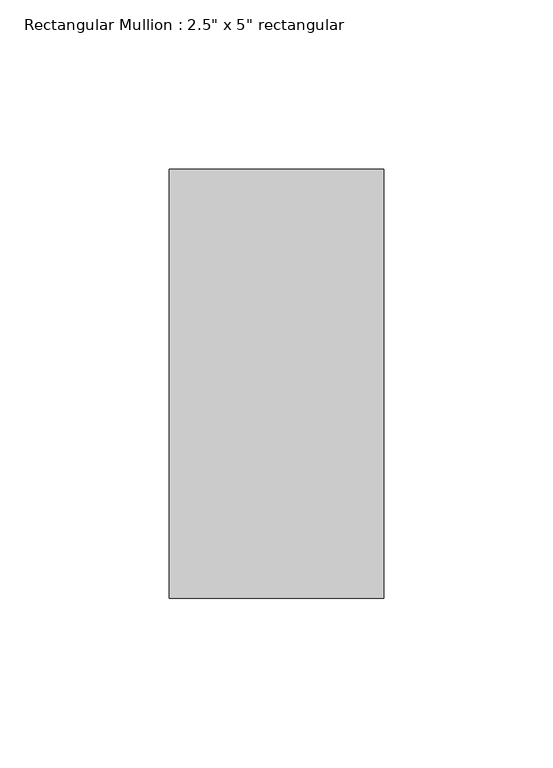
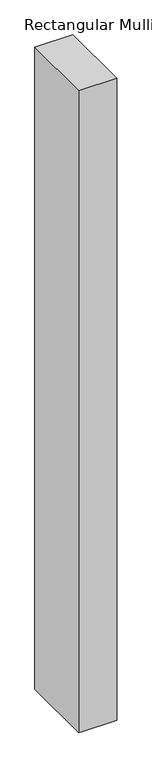
"""IFC4 building model written with IfcOpenShell, lengths in millimetres: member geometry."""

from ifc_helpers import new_model, si_unit, frame, origin, place, context, project, spatial, polyline, outline, extrude, source, transform, mapped, element, save


def member_11cde41b(model_context):
    return source(origin(), model_context, "Body", "SweptSolid", [
        extrude(outline(polyline([(0.0, 63.5), (0.0, -63.5), (-63.5, -63.5), (-63.5, 63.5), (0.0, 63.5)])), frame((0.0, 0.0, -1136.6171844), z_axis=(0.0, 0.0, 1.0), x_axis=(1.0, 0.0, 0.0)), (0.0, 0.0, 1.0), 1136.6171844),
    ])


if __name__ == "__main__":
    model = new_model("IFC4")
    model_context = context("Model", 3, world=origin())
    ifc_project = project(units=[si_unit("LENGTHUNIT", "METRE", prefix="MILLI")], contexts=[model_context])
    site = spatial("IfcSite", under=ifc_project)
    building = spatial("IfcBuilding", under=site)
    placement = place(None, origin())
    member_shape = member_11cde41b(model_context)
    element("IfcMember", 1, ObjectType="Rectangular Mullion : 2.5\" x 5\" rectangular", at=placement, inside=building, context=model_context, shape_type="MappedRepresentation", body=[
        mapped(member_shape, transform((0.0, 0.0, 0.0), x_axis=(1.0, 0.0, 0.0), y_axis=(0.0, 1.0, 0.0), z_axis=(0.0, 0.0, 1.0))),
    ])
    save(model, "model.ifc")

# Revit data of these elements
# Type "Rectangular Mullion : 2.5\" x 5\" rectangular"
#   built-in parameter 1007304 = 0.416667 (stored number, unit not read)
#   built-in parameter 1007301 = 0.104167 (stored number, unit not read)
#   built-in parameter 1007300 = 0.104167 (stored number, unit not read)
# Element 1 (IfcMember, "Rectangular Mullion : 2.5\" x 5\" rectangular")
#   Materials on its faces: "Aluminum"
# Materials
#   "Aluminum": class "Metal", colour RGB 247 247 247, transparency 0, Description = "Aluminum 6061", Cost = 0
